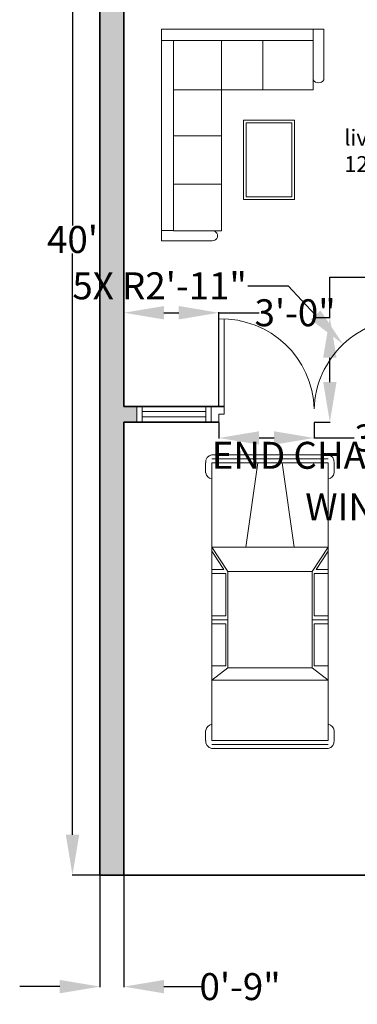
# Model space of a CAD drawing. Units: inches. Extents: x 19 to 15718, y 7 to 930.
# Tile 2 of 11: x 14860 to 14988, y 308 to 680. Entities that reach past the tile are written whole.
import ezdxf

# ---------------------------------------------------------------- set-up
doc = ezdxf.new("R2010")
doc.units = ezdxf.units.IN
doc.header["$MEASUREMENT"] = 0
for name, color, linetype, lineweight in [('A-ANNO-DIMS', 2, 'Continuous', 18), ('A-AREA-IDEN', 7, 'Continuous', 18), ('A-DOOR', 4, 'Continuous', 20), ('A-FURN', 8, 'Continuous', 18), ('A-GLAZ', 4, 'Continuous', 18), ('A-WALL', 7, 'Continuous', 35), ('C-PKNG-VEHC', 8, 'Continuous', 13)]:
    doc.layers.add(name, color=color, linetype=linetype, lineweight=lineweight)
doc.layers.add('A-WALL-PATT', color=18, linetype='Continuous', lineweight=13, true_color=0x000000)
doc.styles.add('Annotative', font='arial.ttf')
doc.styles.get("Standard").update_dxf_attribs({"font": 'arial.ttf'})
doc.dimstyles.get("Standard").update_dxf_attribs({"dimtxt": 10.18, "dimasz": 15.18, "dimexe": 0.18, "dimexo": 0.0625, "dimgap": 0.09, "dimtad": 0, "dimtih": 1, "dimtoh": 1, "dimdec": 0, "dimzin": 0, "dimdsep": 46, "dimlunit": 3, "dimtxsty": 'Standard', "dimcen": 0.09, "dimadec": 0, "dimazin": 0, "dimtfac": 1, "dimtdec": 0, "dimtofl": 0, "dimtmove": 0, "dimatfit": 3, "dimfxl": 1, "dimtolj": 1, "dimtzin": 0, "dimarcsym": 0})

# ---------------------------------------------------------------- blocks, each defined once
blk = doc.blocks.new('*U14')
for p, q in [((5.44, 42.31), (12.12, 42.31)), ((189.69, 42.31), (183.01, 42.31)), ((0.1, -0.41), (0.1, 38.35)), ((2.77, -0.41), (2.77, 38.31)), ((5.44, -0.41), (5.44, 38.24)), ((5.45, 38.31), (16.12, 38.31)), ((16.12, 38.31), (180.34, 38.31)), ((61.52, -0.41), (61.52, 38.31)), ((61.52, 38.31), (77.54, 27.62)), ((64.19, 38.31), (76.2, 30.29)), ((76.2, 30.29), (76.2, 38.31)), ((78.87, 38.31), (78.87, 28.96)), ((106.91, 28.96), (106.91, 38.31)), ((109.58, 27.62), (109.58, 38.31)), ((112.25, 38.31), (112.25, 28.96)), ((140.29, 28.96), (140.29, 38.31)), ((141.62, 27.62), (149.64, 38.31)), ((149.64, -0.41), (149.64, 38.31)), ((189.69, 38.31), (179.01, 38.31)), ((189.69, -0.41), (189.69, 38.24)), ((192.36, -0.41), (192.36, 38.31)), ((195.03, -0.41), (195.03, 38.35)), ((77.54, 27.62), (141.62, 27.62)), ((77.54, -0.41), (77.54, 27.62)), ((78.87, 28.96), (106.91, 28.96)), ((112.25, 28.96), (140.29, 28.96)), ((141.62, -0.41), (141.62, 27.62)), ((5.44, 7.6), (61.52, 15.61)), ((0.1, -0.42), (0.1, -39.18)), ((2.77, -0.41), (2.77, -39.13)), ((5.44, -0.42), (5.44, -39.07)), ((61.52, -0.41), (61.52, -39.13)), ((77.54, -0.41), (77.54, -28.45)), ((141.62, -0.41), (141.62, -28.45)), ((149.64, -0.41), (149.64, -39.13)), ((189.69, -0.42), (189.69, -39.07)), ((192.36, -0.41), (192.36, -39.13)), ((195.03, -0.42), (195.03, -39.18)), ((5.44, -8.42), (61.52, -16.43)), ((61.52, -39.13), (77.54, -28.45)), ((64.19, -39.13), (76.2, -31.12)), ((76.2, -31.12), (76.2, -39.13)), ((77.54, -28.45), (141.62, -28.45)), ((78.87, -39.13), (78.87, -29.79)), ((78.87, -29.79), (106.91, -29.79)), ((106.91, -29.79), (106.91, -39.13)), ((109.58, -28.45), (109.58, -39.13)), ((112.25, -29.79), (140.29, -29.79)), ((112.25, -39.13), (112.25, -29.79)), ((140.29, -29.79), (140.29, -39.13)), ((141.62, -28.45), (149.64, -39.13)), ((5.45, -39.13), (16.12, -39.13)), ((16.12, -39.13), (180.34, -39.13)), ((189.69, -39.13), (179.01, -39.13)), ((5.44, -43.14), (12.12, -43.14)), ((189.69, -43.14), (183.01, -43.14))]:
    blk.add_line(p, q)
for centre, radius, start, end in [((5.06, 37.26), 5.06, 85.64554, 168.0943), ((11.45, 37.64), 4.72, 8.13011, 81.86996), ((183.68, 37.64), 4.72, 98.13004, 171.8699), ((190.07, 37.26), 5.06, 11.90574, 94.35446), ((5.06, -38.09), 5.06, 191.9057, 274.3545), ((11.45, -38.46), 4.72, 278.13, 351.8699), ((183.68, -38.46), 4.72, 188.1301, 261.87), ((190.07, -38.09), 5.06, 265.6455, 348.0943)]:
    blk.add_arc(centre, radius, start, end)
blk = doc.blocks.new('*D6')
at = {"layer": 'A-ANNO-DIMS', "color": 0, "lineweight": -2, "transparency": 16777216}
for p, q in [((14890.77, 837.06), (14880.28, 837.06)), ((14880.46, 821.88), (14880.46, 602.31)), ((14880.46, 372.18), (14880.46, 591.74)), ((14890.77, 357), (14880.28, 357))]:
    blk.add_line(p, q, dxfattribs=at)
at = {"layer": 'A-ANNO-DIMS', "color": 0, "transparency": 16777216}
for points in [[(14877.93, 821.88), (14882.99, 821.88), (14880.46, 837.06)], [(14877.93, 372.18), (14882.99, 372.18), (14880.46, 357)]]:
    blk.add_solid(points, dxfattribs=at)
at = {"layer": 'Defpoints', "color": 0, "transparency": 16777216}
for p in [(14890.84, 837.06), (14880.46, 357), (14890.84, 357)]:
    blk.add_point(p, dxfattribs=at)
at = {"layer": 'A-ANNO-DIMS', "color": 0, "transparency": 16777216, "insert": (14880.46, 597.03), "char_height": 10.18, "attachment_point": 5}
blk.add_mtext("\\A1;40'", dxfattribs=at)
blk = doc.blocks.new('DOOR-ENTRY-LEAF-36IN')
for p, q in [((0, 6), (0, 39)), ((2, 3), (2, 39)), ((0, 3), (0, 0)), ((2, 3), (0, 3))]:
    blk.add_line(p, q)
blk.add_arc((1, 4), 35.01, 1.6366, 91.6366)
blk = doc.blocks.new('WIN-24IN-FRAME6')
for p, q in [((0, 28), (6, 28)), ((0, 26), (6, 26)), ((2, 26), (2, 2)), ((4, 26), (4, 2)), ((0, 2), (6, 2)), ((0, 0), (6, 0))]:
    blk.add_line(p, q)
blk = doc.blocks.new('*D36')
at = {"layer": 'A-ANNO-DIMS', "color": 0, "lineweight": -2, "transparency": 16777216}
for p, q in [((15054.04, 525.18), (15054.04, 540.36)), ((15049.9, 510), (15054.22, 510)), ((15049.9, 482), (15054.22, 482)), ((15054.04, 466.82), (15054.04, 451.64))]:
    blk.add_line(p, q, dxfattribs=at)
at = {"layer": 'A-ANNO-DIMS', "color": 0, "transparency": 16777216}
for points in [[(15051.51, 525.18), (15056.57, 525.18), (15054.04, 510)], [(15051.51, 466.82), (15056.57, 466.82), (15054.04, 482)]]:
    blk.add_solid(points, dxfattribs=at)
at = {"layer": 'Defpoints', "color": 0, "transparency": 16777216}
for p in [(15049.84, 510), (15054.04, 510), (15049.84, 482)]:
    blk.add_point(p, dxfattribs=at)
at = {"layer": 'A-ANNO-DIMS', "color": 0, "transparency": 16777216, "insert": (15054.04, 496), "char_height": 10.18, "attachment_point": 5}
blk.add_mtext('\\A1;WINDOW FRAME 2\'-4" TYP.', dxfattribs=at)
blk = doc.blocks.new('*D50')
at = {"layer": 'A-ANNO-DIMS', "color": 0, "lineweight": -2, "transparency": 16777216}
for p, q in [((14977.77, 567.55), (14977.77, 582.73)), ((14977.77, 582.73), (14992.95, 582.73)), ((14971.9, 567.55), (14977.95, 567.55)), ((14977.77, 543.18), (14977.77, 552.37)), ((14971.9, 528), (14977.95, 528))]:
    blk.add_line(p, q, dxfattribs=at)
at = {"layer": 'A-ANNO-DIMS', "color": 0, "transparency": 16777216}
for points in [[(14975.24, 552.37), (14980.3, 552.37), (14977.77, 567.55)], [(14975.24, 543.18), (14980.3, 543.18), (14977.77, 528)]]:
    blk.add_solid(points, dxfattribs=at)
at = {"layer": 'Defpoints', "color": 0, "transparency": 16777216}
for p in [(14971.84, 567.55), (14977.77, 567.55), (14971.84, 528)]:
    blk.add_point(p, dxfattribs=at)
at = {"layer": 'A-ANNO-DIMS', "color": 0, "transparency": 16777216, "insert": (15081.49, 582.73), "char_height": 10.18, "attachment_point": 5}
blk.add_mtext('\\A1;ENTRY LEAF 3\'-3 1/2" TYP.', dxfattribs=at)
blk = doc.blocks.new('*D51')
at = {"layer": 'A-ANNO-DIMS', "color": 0, "lineweight": -2, "transparency": 16777216}
for p, q in [((14935.84, 527.93), (14935.84, 521.88)), ((14971.84, 527.93), (14971.84, 521.88)), ((14951.02, 522.06), (14956.66, 522.06)), ((14971.84, 522.06), (14987.02, 522.06))]:
    blk.add_line(p, q, dxfattribs=at)
at = {"layer": 'A-ANNO-DIMS', "color": 0, "transparency": 16777216}
for points in [[(14951.02, 524.59), (14951.02, 519.53), (14935.84, 522.06)], [(14956.66, 524.59), (14956.66, 519.53), (14971.84, 522.06)]]:
    blk.add_solid(points, dxfattribs=at)
at = {"layer": 'Defpoints', "color": 0, "transparency": 16777216}
for p in [(14935.84, 528), (14971.84, 528), (14971.84, 522.06)]:
    blk.add_point(p, dxfattribs=at)
at = {"layer": 'A-ANNO-DIMS', "color": 0, "transparency": 16777216, "insert": (15018.13, 522.06), "char_height": 10.18, "attachment_point": 5}
blk.add_mtext('\\A1;3\'-0" TYP.', dxfattribs=at)
blk = doc.blocks.new('*D54')
at = {"layer": 'A-ANNO-DIMS', "color": 0, "lineweight": -2, "transparency": 16777216}
for p, q in [((15112.3, 568.4), (15112.3, 583.58)), ((15111.26, 553.22), (15112.48, 553.22)), ((15111.26, 545.87), (15112.48, 545.87)), ((15112.3, 530.69), (15112.3, 515.51)), ((15112.3, 515.51), (15097.12, 515.51))]:
    blk.add_line(p, q, dxfattribs=at)
at = {"layer": 'A-ANNO-DIMS', "color": 0, "transparency": 16777216}
for points in [[(15109.77, 568.4), (15114.83, 568.4), (15112.3, 553.22)], [(15109.77, 530.69), (15114.83, 530.69), (15112.3, 545.87)]]:
    blk.add_solid(points, dxfattribs=at)
at = {"layer": 'Defpoints', "color": 0, "transparency": 16777216}
for p in [(15111.2, 553.22), (15111.2, 545.87), (15112.3, 545.87)]:
    blk.add_point(p, dxfattribs=at)
at = {"layer": 'A-ANNO-DIMS', "color": 0, "transparency": 16777216, "insert": (15013.32, 515.51), "char_height": 10.18, "attachment_point": 5}
blk.add_mtext('\\A1;END CHAIR 0\'-7 1/2" TYP.', dxfattribs=at)
blk = doc.blocks.new('*D83')
at = {"layer": 'A-ANNO-DIMS', "color": 0, "lineweight": -2, "transparency": 16777216}
for p, q in [((14890.84, 356.93), (14890.84, 314.67)), ((14899.84, 356.93), (14899.84, 314.67)), ((14875.66, 314.85), (14860.48, 314.85)), ((14915.02, 314.85), (14930.2, 314.85))]:
    blk.add_line(p, q, dxfattribs=at)
at = {"layer": 'A-ANNO-DIMS', "color": 0, "transparency": 16777216}
for points in [[(14875.66, 317.38), (14875.66, 312.32), (14890.84, 314.85)], [(14915.02, 317.38), (14915.02, 312.32), (14899.84, 314.85)]]:
    blk.add_solid(points, dxfattribs=at)
at = {"layer": 'Defpoints', "color": 0, "transparency": 16777216}
for p in [(14890.84, 357), (14899.84, 357), (14899.84, 314.85)]:
    blk.add_point(p, dxfattribs=at)
at = {"layer": 'A-ANNO-DIMS', "color": 0, "transparency": 16777216, "insert": (14943.82, 314.85), "char_height": 10.18, "attachment_point": 5}
blk.add_mtext('\\A1;0\'-9"', dxfattribs=at)
blk = doc.blocks.new('*D84')
at = {"layer": 'A-ANNO-DIMS', "color": 0, "lineweight": -2, "transparency": 16777216}
for p, q in [((14899.84, 534.06), (14899.84, 569.53)), ((14915.02, 569.35), (14920.66, 569.35)), ((14935.84, 534.06), (14935.84, 569.53)), ((14935.84, 569.35), (14951.02, 569.35))]:
    blk.add_line(p, q, dxfattribs=at)
at = {"layer": 'A-ANNO-DIMS', "color": 0, "transparency": 16777216}
for points in [[(14915.02, 571.88), (14915.02, 566.82), (14899.84, 569.35)], [(14920.66, 571.88), (14920.66, 566.82), (14935.84, 569.35)]]:
    blk.add_solid(points, dxfattribs=at)
at = {"layer": 'Defpoints', "color": 0, "transparency": 16777216}
for p in [(14935.84, 569.35), (14899.84, 534), (14935.84, 534)]:
    blk.add_point(p, dxfattribs=at)
at = {"layer": 'A-ANNO-DIMS', "color": 0, "transparency": 16777216, "insert": (14964.63, 569.35), "char_height": 10.18, "attachment_point": 5}
blk.add_mtext('\\A1;3\'-0"', dxfattribs=at)
blk = doc.blocks.new('*D87')
at = {"layer": 'A-ANNO-DIMS', "color": 0, "lineweight": -2, "transparency": 16777216}
for p, q in [((14946.77, 579.52), (14961.95, 579.52)), ((14961.95, 579.52), (14972.37, 568.49)), ((15006.75, 532), (15006.93, 532)), ((15006.84, 531.91), (15006.84, 532.09))]:
    blk.add_line(p, q, dxfattribs=at)
at = {"layer": 'A-ANNO-DIMS', "color": 0, "transparency": 16777216}
blk.add_solid([(14974.21, 570.22), (14970.53, 566.75), (14982.79, 557.45)], dxfattribs=at)
at = {"layer": 'Defpoints', "color": 0, "transparency": 16777216}
for p in [(14982.79, 557.45), (15006.84, 532)]:
    blk.add_point(p, dxfattribs=at)
at = {"layer": 'A-ANNO-DIMS', "color": 0, "transparency": 16777216, "insert": (14913.39, 579.52), "char_height": 10.18, "attachment_point": 5}
blk.add_mtext('\\A1;5X R2\'-11"', dxfattribs=at)

msp = doc.modelspace()

# ---------------------------------------------------------------- hatches: boundary and pattern name
at = {"layer": 'A-WALL-PATT'}
h = msp.add_hatch(color=256, dxfattribs=at)
h.dxf.hatch_style = 1
h.paths.add_polyline_path([(15190.84, 837), (14890.84, 837), (14890.84, 357), (14899.84, 357), (14899.84, 366), (14899.84, 528), (14904.84, 528), (14904.84, 534), (14899.84, 534), (14899.84, 698), (15004.84, 698), (15004.84, 701, -0.014283), (15004.84, 703), (15004.84, 704), (14899.84, 704), (14899.84, 828), (14987.26, 828), (15043.84, 828), (15049.84, 828), (15075.84, 828), (15081.84, 828), (15181.84, 828), (15181.84, 780), (15114.84, 780), (15114.84, 779, -0.017236), (15114.84, 777), (15114.84, 774), (15181.84, 774), (15181.84, 654), (15181.84, 648), (15181.84, 596), (15190.84, 596)])
h.paths.add_polyline_path([(15190.84, 590), (15181.84, 590), (15181.84, 470), (15181.84, 464), (15181.84, 361.43), (14991.9, 361.43), (14991.5, 357), (15190.84, 357)], flags=0)
h.paths.add_polyline_path([(15152.29, 608), (15146.29, 608), (15146.29, 596), (15049.84, 596), (15049.84, 590), (15152.29, 590)], flags=17)
h.paths.add_polyline_path([(15049.84, 615), (15048.84, 615, -0.017236), (15046.84, 615), (15043.84, 615), (15043.84, 596), (15049.84, 596)], flags=17)
edge = h.paths.add_edge_path(flags=17)
edge.add_line((15152.29, 654), (15049.84, 654))
edge.add_line((15049.84, 654), (15043.84, 654))
edge.add_line((15043.84, 654), (15043.84, 648))
edge.add_line((15043.84, 648), (15049.84, 648))
edge.add_line((15049.84, 648), (15075.84, 648))
edge.add_line((15075.84, 648), (15081.84, 648))
edge.add_line((15081.84, 648), (15117.26, 648))
edge.add_spline(control_points=[(15117.26, 648), (15117.59, 648.02), (15117.94, 648.03), (15118.71, 648.04), (15119.15, 648.02), (15119.59, 648)], knot_values=[1.499122, 1.499122, 1.499122, 1.499122, 1.618335, 1.618335, 1.770388, 1.770388, 1.770388, 1.770388], degree=3, periodic=0)
edge.add_spline(control_points=[(15127.99, 642.93), (15128, 643.28), (15127.95, 643.62), (15127.73, 644.26), (15127.57, 644.57), (15127.16, 645.13), (15126.92, 645.39), (15126.04, 646.16), (15125.28, 646.6), (15123.53, 647.31), (15122.55, 647.59), (15120.88, 647.88), (15120.24, 647.95), (15119.59, 648)], knot_values=[0, 0, 0, 0, 0.172075, 0.172075, 0.344149, 0.344149, 0.516224, 0.516224, 0.894541, 0.894541, 1.272858, 1.272858, 1.499122, 1.499122, 1.499122, 1.499122], degree=3, periodic=0)
edge.add_line((15119.59, 648), (15146.29, 648))
edge.add_line((15146.29, 648), (15146.29, 636))
edge.add_line((15146.29, 636), (15152.29, 636))
edge.add_line((15152.29, 636), (15152.29, 654))
h.paths.add_polyline_path([(15132.35, 430.4), (15123.35, 430.4), (15123.35, 396.8), (15027.77, 396.8), (15027.77, 387.8), (15132.35, 387.8)], flags=17)
h.paths.add_polyline_path([(15132.35, 464), (15123.35, 464), (15123.35, 430.4), (15132.35, 430.4)], flags=17)
h.paths.add_polyline_path([(15275.68, 583.59), (15276.07, 583.2), (15276.65, 583.2), (15280.6, 587.16), (15278.55, 589.2), (15275.68, 589.2), (15275.68, 601.2), (15266.68, 601.2), (15266.68, 350.2), (15275.68, 350.2), (15275.68, 359.2), (15275.68, 457.2), (15413.68, 457.2), (15413.68, 471.04), (15407.68, 471.04), (15407.68, 463.2), (15275.68, 463.2)])

# ---------------------------------------------------------------- linework, layer by layer
at = {"layer": 'A-DOOR'}
for p, q in [((14971.79, 534), (14971.88, 534)), ((14971.84, 534), (14971.84, 533))]:
    msp.add_line(p, q, dxfattribs=at)
msp.add_arc((15006.84, 532), 35.01, 88.3634, 178.3634, dxfattribs=at)
at = {"layer": 'A-FURN'}
for p, q in [((14952.37, 653.54), (14952.37, 672.13)), ((14918.66, 636.2), (14936.77, 636.2)), ((14918.66, 617.86), (14936.77, 617.86))]:
    msp.add_line(p, q, dxfattribs=at)
for points in [[(14914.12, 672.13), (14971.51, 672.13), (14971.51, 676.46), (14914.12, 676.46)], [(14918.66, 672.13), (14914.12, 672.13), (14914.12, 600.41), (14918.66, 600.41)], [(14918.66, 600.27), (14936.77, 600.27), (14936.77, 672.13), (14918.66, 672.13)], [(14918.66, 672.13), (14971.49, 672.13), (14971.49, 653.54), (14918.66, 653.54)], [(14945.13, 642.13), (14964.38, 642.13), (14964.38, 612.1), (14945.13, 612.1)], [(14946.13, 641.13), (14963.38, 641.13), (14963.38, 613.1), (14946.13, 613.1)]]:
    msp.add_lwpolyline(points, close=True, dxfattribs=at)
for points in [[(14971.51, 657.28), (14971.51, 676.46), (14975.5, 676.46), (14975.5, 657.28)], [(14933.25, 596.57), (14914.12, 596.57), (14914.12, 600.41), (14918.66, 600.41)]]:
    msp.add_lwpolyline(points, dxfattribs=at)
for centre, radius, start, end in [((14973.51, 658.52), 2.35, 211.8626, 328.1374), ((14933.47, 598.42), 1.86, 263.3439, 96.6561)]:
    msp.add_arc(centre, radius, start, end, dxfattribs=at)
at = {"layer": 'A-WALL'}
for p, q in [((14890.84, 357), (14890.84, 837)), ((14899.84, 534), (14899.84, 698)), ((14899.84, 534), (14937.84, 534)), ((14899.84, 366), (14899.84, 528)), ((14899.84, 528), (14935.84, 528)), ((14899.84, 366), (14899.84, 357)), ((15190.84, 357), (14890.84, 357))]:
    msp.add_line(p, q, dxfattribs=at)

# ---------------------------------------------------------------- block references
at = {"layer": 'A-DOOR'}
msp.add_blockref('DOOR-ENTRY-LEAF-36IN', (14935.84, 528), dxfattribs=at)
at = {"layer": 'A-GLAZ', "rotation": 270.0000000000164}
msp.add_blockref('WIN-24IN-FRAME6', (14904.84, 534), dxfattribs=at)
at = {"layer": 'C-PKNG-VEHC', "xscale": 0.5691226359303588, "yscale": 0.5691226359303588, "zscale": 0.5691226359303588, "rotation": 270}
msp.add_blockref('*U14', (14955.36, 515.79), dxfattribs=at)

# ---------------------------------------------------------------- texts
at = {"layer": 'A-AREA-IDEN', "insert": (14983.24, 638.5), "char_height": 6, "width": 68.1983, "attachment_point": 1, "style": 'Annotative'}
msp.add_mtext('living\\P12\'4"x13\'8"', dxfattribs=at)

# ---------------------------------------------------------------- dimensions: what is measured, and where the dimension line sits
at = {"layer": 'A-ANNO-DIMS'}
dim = msp.add_linear_dim(base=(14880.46, 357), p1=(14890.84, 837.06), p2=(14890.84, 357), angle=90, dimstyle='Standard', override={"dimclrd": 0, "dimclre": 0, "dimclrt": 0}, dxfattribs=at)
dim.commit()
dim.dimension.update_dxf_attribs({"geometry": '*D6', "text_midpoint": (14880.46, 597.03)})
for base, p1, p2, angle, text, picture, middle in [((14977.7695, 567.5479), (14971.8366, 527.9956), (14971.8366, 567.5479), 90, 'ENTRY LEAF <> TYP.', '*D50', (15081.493, 582.7279)), ((15112.3017, 545.8656), (15111.1988, 553.2183), (15111.1988, 545.8656), 270, 'END CHAIR <> TYP.', '*D54', (15013.3244, 515.5056)), ((15054.04, 510), (15049.84, 482), (15049.84, 510), 90, 'WINDOW FRAME <> TYP.', '*D36', (15054.04, 496))]:
    dim = msp.add_linear_dim(base=base, p1=p1, p2=p2, angle=angle, text=text, dimstyle='Standard', override={"dimdec": 1, "dimlfac": 1, "dimrnd": 0, "dimzin": 1, "dimdsep": 46, "dimlunit": 4, "dimfrac": 2}, dxfattribs=at)
    dim.commit()
    dim.dimension.update_dxf_attribs({"geometry": picture, "text_midpoint": middle})
dim = msp.add_radius_dim(center=(15006.84, 532), mpoint=(14982.79, 557.45), text='5X <>', dimstyle='Standard', override={"dimdec": 1, "dimlfac": 1, "dimrnd": 0, "dimzin": 1, "dimdsep": 46, "dimlunit": 4, "dimfrac": 2}, dxfattribs=at)
dim.commit()
dim.dimension.update_dxf_attribs({"geometry": '*D87', "text_midpoint": (14913.39, 579.52)})
for base, p1, p2, picture, middle in [((14935.84, 569.35), (14899.84, 534), (14935.84, 534), '*D84', (14964.63, 569.35)), ((14899.84, 314.85), (14890.84, 357), (14899.84, 357), '*D83', (14943.82, 314.85))]:
    dim = msp.add_linear_dim(base=base, p1=p1, p2=p2, dimstyle='Standard', override={"dimdec": 1, "dimlfac": 1, "dimrnd": 0, "dimzin": 1, "dimdsep": 46, "dimlunit": 4, "dimfrac": 2}, dxfattribs=at)
    dim.commit()
    dim.dimension.update_dxf_attribs({"geometry": picture, "text_midpoint": middle})
dim = msp.add_linear_dim(base=(14971.84, 522.06), p1=(14935.84, 528), p2=(14971.84, 528), text='<> TYP.', dimstyle='Standard', override={"dimdec": 1, "dimlfac": 1, "dimrnd": 0, "dimzin": 1, "dimdsep": 46, "dimlunit": 4, "dimfrac": 2}, dxfattribs=at)
dim.commit()
dim.dimension.update_dxf_attribs({"geometry": '*D51', "text_midpoint": (15018.13, 522.06)})

doc.saveas('drawing.dxf')
